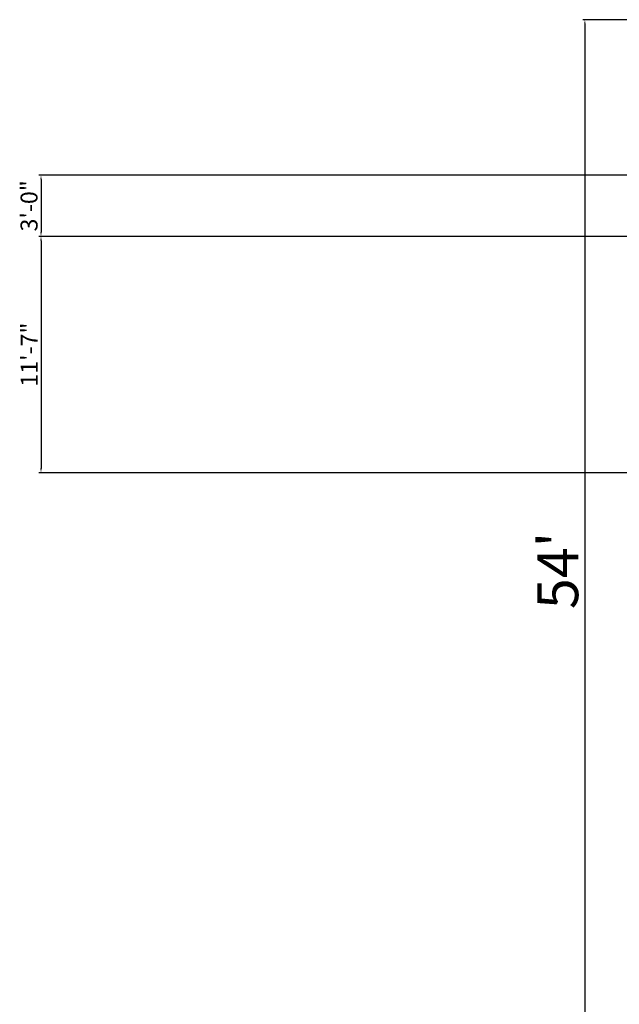
# Model space of a CAD drawing. Units: inches. Extents: x 2214 to 3937, y 762 to 2085.
# Tile 2 of 9: x 2214 to 2567, y 1424 to 2003. Entities that reach past the tile are written whole.
import ezdxf

# ---------------------------------------------------------------- set-up
doc = ezdxf.new("R2010")
doc.units = ezdxf.units.IN
doc.layers.add('C-ANNO-DIMS', color=2, linetype='Continuous', lineweight=18)
doc.styles.get("Standard").update_dxf_attribs({"font": 'arial.ttf'})
doc.dimstyles.new('ISO-25', dxfattribs={"dimtxt": 10, "dimasz": 2.5, "dimexe": 1.25, "dimexo": 0.625, "dimtad": 1, "dimdec": 1, "dimlunit": 4, "dimtxsty": 'Standard', "dimcen": 2.5, "dimadec": 0, "dimazin": 0, "dimtfac": 1, "dimtdec": 1, "dimtmove": 0, "dimatfit": 3, "dimfxl": 1, "dimarcsym": 0})

# ---------------------------------------------------------------- blocks, each defined once
blk = doc.blocks.new('*D20')
at = {"layer": 'C-ANNO-DIMS', "color": 0, "lineweight": -2, "ltscale": 0.3, "transparency": 16777216}
for p, q in [((2581.93, 2003.22), (2545.31, 2003.22)), ((2546.56, 2000.72), (2546.56, 1357.72)), ((2581.93, 1355.22), (2545.31, 1355.22))]:
    blk.add_line(p, q, dxfattribs=at)
at = {"layer": 'C-ANNO-DIMS', "color": 0, "ltscale": 0.3, "transparency": 16777216}
for points in [[(2546.14, 2000.72), (2546.97, 2000.72), (2546.56, 2003.22)], [(2546.14, 1357.72), (2546.97, 1357.72), (2546.56, 1355.22)]]:
    blk.add_solid(points, dxfattribs=at)
at = {"layer": 'Defpoints', "color": 0, "ltscale": 0.3, "transparency": 16777216}
for p in [(2582.56, 2003.22), (2546.56, 1355.22), (2582.56, 1355.22)]:
    blk.add_point(p, dxfattribs=at)
at = {"layer": 'C-ANNO-DIMS', "color": 0, "ltscale": 0.3, "transparency": 16777216, "insert": (2533.73, 1679.22), "char_height": 24, "attachment_point": 5, "rotation": 90}
blk.add_mtext("54'", dxfattribs=at)
blk = doc.blocks.new('*D62')
at = {"layer": 'C-ANNO-DIMS', "color": 0, "lineweight": -2, "ltscale": 0.3, "transparency": 16777216}
for p, q in [((3240.43, 1911.72), (2225.23, 1911.72)), ((2226.48, 1909.22), (2226.48, 1878.22)), ((3240.43, 1875.72), (2225.23, 1875.72))]:
    blk.add_line(p, q, dxfattribs=at)
at = {"layer": 'C-ANNO-DIMS', "color": 0, "ltscale": 0.3, "transparency": 16777216}
for points in [[(2226.07, 1909.22), (2226.9, 1909.22), (2226.48, 1911.72)], [(2226.07, 1878.22), (2226.9, 1878.22), (2226.48, 1875.72)]]:
    blk.add_solid(points, dxfattribs=at)
at = {"layer": 'Defpoints', "color": 0, "ltscale": 0.3, "transparency": 16777216}
for p in [(3241.06, 1911.72), (2226.48, 1875.72), (3241.06, 1875.72)]:
    blk.add_point(p, dxfattribs=at)
at = {"layer": 'C-ANNO-DIMS', "color": 0, "ltscale": 0.3, "transparency": 16777216, "insert": (2220.75, 1893.72), "char_height": 10, "attachment_point": 5, "rotation": 90}
blk.add_mtext('3\'-0"', dxfattribs=at)
blk = doc.blocks.new('*D63')
at = {"layer": 'C-ANNO-DIMS', "color": 0, "lineweight": -2, "ltscale": 0.3, "transparency": 16777216}
for p, q in [((3240.43, 1875.72), (2225.23, 1875.72)), ((2226.48, 1873.22), (2226.48, 1739.22)), ((3240.43, 1736.72), (2225.23, 1736.72))]:
    blk.add_line(p, q, dxfattribs=at)
at = {"layer": 'C-ANNO-DIMS', "color": 0, "ltscale": 0.3, "transparency": 16777216}
for points in [[(2226.07, 1873.22), (2226.9, 1873.22), (2226.48, 1875.72)], [(2226.07, 1739.22), (2226.9, 1739.22), (2226.48, 1736.72)]]:
    blk.add_solid(points, dxfattribs=at)
at = {"layer": 'Defpoints', "color": 0, "ltscale": 0.3, "transparency": 16777216}
for p in [(3241.06, 1875.72), (2226.48, 1736.72), (3241.06, 1736.72)]:
    blk.add_point(p, dxfattribs=at)
at = {"layer": 'C-ANNO-DIMS', "color": 0, "ltscale": 0.3, "transparency": 16777216, "insert": (2220.84, 1806.22), "char_height": 10, "attachment_point": 5, "rotation": 90}
blk.add_mtext('11\'-7"', dxfattribs=at)

msp = doc.modelspace()

# ---------------------------------------------------------------- dimensions: what is measured, and where the dimension line sits
at = {"layer": 'C-ANNO-DIMS', "ltscale": 0.3}
for base, p1, p2, override, picture, middle in [((2546.56, 1355.22), (2582.56, 2003.22), (2582.56, 1355.22), {"dimtxt": 24, "dimclrd": 0, "dimclre": 0, "dimclrt": 0}, '*D20', (2533.73, 1679.22)), ((2226.48, 1875.72), (3241.06, 1911.72), (3241.06, 1875.72), {"dimdec": 1, "dimlfac": 1, "dimrnd": 0, "dimzin": 1, "dimdsep": 46, "dimlunit": 4, "dimfrac": 2}, '*D62', (2220.75, 1893.72)), ((2226.48, 1736.72), (3241.06, 1875.72), (3241.06, 1736.72), {"dimdec": 1, "dimlfac": 1, "dimrnd": 0, "dimzin": 1, "dimdsep": 46, "dimlunit": 4, "dimfrac": 2}, '*D63', (2220.84, 1806.22))]:
    dim = msp.add_linear_dim(base=base, p1=p1, p2=p2, angle=90, dimstyle='ISO-25', override=override, dxfattribs=at)
    dim.commit()
    dim.dimension.update_dxf_attribs({"geometry": picture, "text_midpoint": middle})

doc.saveas('drawing.dxf')
